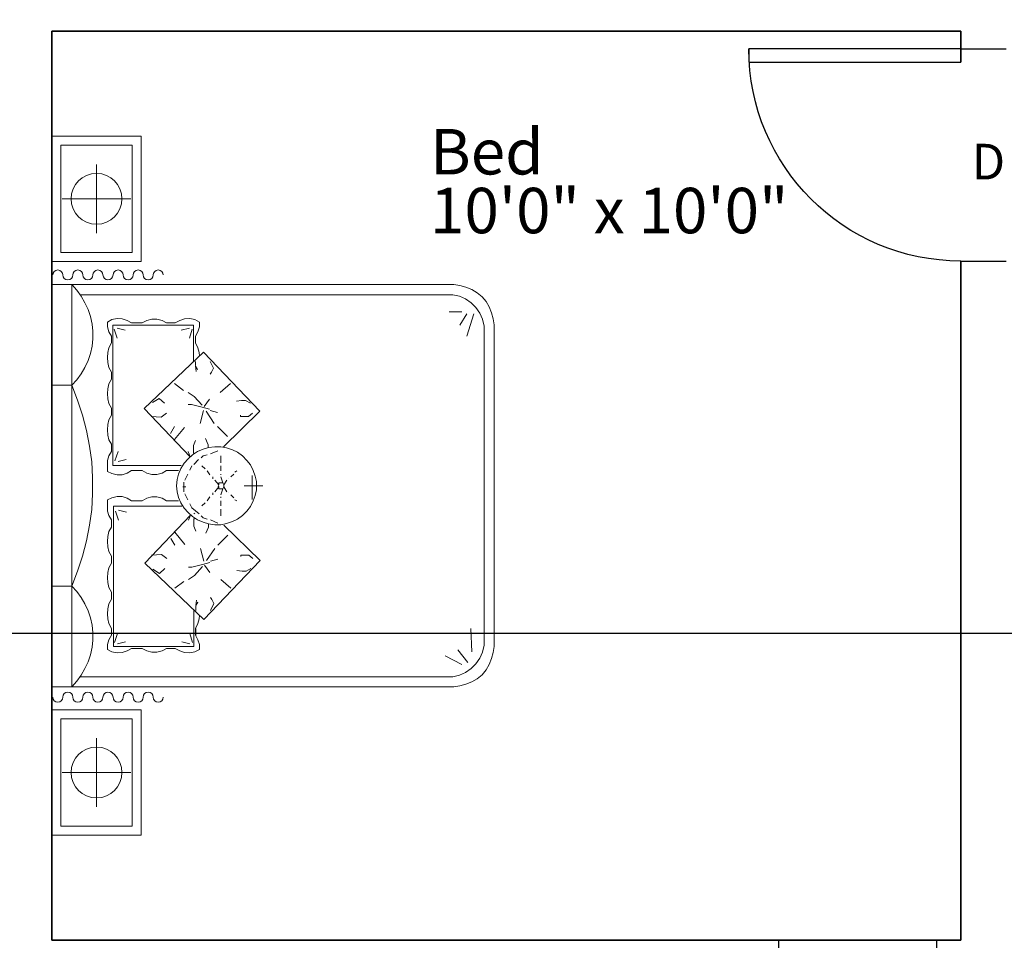
# Model space of a CAD drawing. Units: inches. Extents: x -1198 to -69, y -512 to 437.
# Tile 27 of 50: x -696 to -566, y -85 to 37. Entities that reach past the tile are written whole.
import ezdxf

# ---------------------------------------------------------------- set-up
doc = ezdxf.new("R2010")
doc.units = ezdxf.units.IN
doc.header["$MEASUREMENT"] = 0
for name, color, linetype, lineweight in [('A-ANNO-DIMS', 2, 'Continuous', 18), ('A-ANNO-SYMB', 7, 'Continuous', 18), ('A-AREA-IDEN', 7, 'Continuous', 18), ('A-FURN', 60, 'Continuous', 18), ('A-WALL', 7, 'Continuous', 35), ('Doors', 140, 'Continuous', 25), ('ds_furniture_Pen_No__7', 7, 'Continuous', 18)]:
    doc.layers.add(name, color=color, linetype=linetype, lineweight=lineweight)
doc.styles.get("Standard").update_dxf_attribs({"font": 'arial.ttf'})
doc.dimstyles.get("Standard").update_dxf_attribs({"dimtxt": 6, "dimasz": 6, "dimexe": 0.18, "dimexo": 0.0625, "dimgap": 0.09, "dimtad": 0, "dimtih": 1, "dimtoh": 1, "dimdec": 0, "dimzin": 0, "dimdsep": 46, "dimlunit": 4, "dimtxsty": 'Standard', "dimblk": 'OBLIQUE', "dimcen": 0.09, "dimadec": 0, "dimazin": 0, "dimtfac": 1, "dimtdec": 0, "dimtofl": 0, "dimtmove": 0, "dimatfit": 3, "dimfxl": 1, "dimtolj": 1, "dimtzin": 0, "dimarcsym": 0})

# ---------------------------------------------------------------- blocks, each defined once
blk = doc.blocks.new('*U4')
for p, q in [((0, 0), (0, -6)), ((28, 0), (28, -6))]:
    blk.add_line(p, q)
blk.add_lwpolyline([(0, 0), (0, 28), (1.75, 28), (1.75, 0)], close=True)
blk.add_arc((0, 0), 28, 0, 90)
blk = doc.blocks.new('new')
at = {"layer": 'ds_furniture_Pen_No__7'}
for p, q in [((-1180, 2274.4), (-1838.2, 2274.4)), ((-1838.2, 2274.4), (-1838.2, 1804.2)), ((-1180, 1804.2), (-1180, 2274.4)), ((-1057.8, 158.7), (-1057.8, 2274.4)), ((-1057.8, 2274.4), (1057.8, 2274.4)), ((-1057.8, 2274.4), (1057.8, 2274.4)), ((-1057.8, 158.7), (-1057.8, 2274.4)), ((-528.9, 2274.4), (-528.9, 2168.6)), ((528.9, 2274.4), (528.9, 2168.6)), ((1057.8, 2274.4), (1057.8, 158.7)), ((1057.8, 2274.4), (1057.8, 158.7)), ((1180, 1804.2), (1180, 2274.4)), ((1180, 2274.4), (1838.2, 2274.4)), ((1838.2, 2274.4), (1838.2, 1804.2)), ((-1227, 2227.4), (-1791.2, 2227.4)), ((-1791.2, 2227.4), (-1791.2, 1851.2)), ((-1509.1, 2220.2), (-1509.1, 1858.4)), ((-1227, 1851.2), (-1227, 2227.4)), ((1227, 1851.2), (1227, 2227.4)), ((1227, 2227.4), (1791.2, 2227.4)), ((1509.1, 2220.2), (1509.1, 1858.4)), ((1791.2, 2227.4), (1791.2, 1851.2)), ((1057.8, 2168.6), (-1057.8, 2168.6)), ((-1057.8, 2168.6), (-1028.2, 2143.2)), ((-1028.2, 2143.2), (-996.5, 2119.9)), ((-588.2, 2119.9), (-556.4, 2143.2)), ((-556.4, 2143.2), (-528.9, 2168.6)), ((-528.9, 2168.6), (-450.6, 2139)), ((-450.6, 2139), (-370.2, 2113.6)), ((370.2, 2113.6), (450.6, 2139)), ((450.6, 2139), (528.9, 2168.6)), ((528.9, 2168.6), (556.4, 2143.2)), ((556.4, 2143.2), (588.2, 2119.9)), ((996.5, 2119.9), (1028.2, 2143.2)), ((1028.2, 2143.2), (1057.8, 2168.6)), ((-1005, 165), (-1005, 2124.2)), ((-996.5, 2119.9), (-962.6, 2100.9)), ((-962.6, 2100.9), (-926.7, 2084)), ((-926.7, 2084), (-890.7, 2071.3)), ((-696.1, 2071.3), (-658, 2084)), ((-658, 2084), (-622, 2100.9)), ((-622, 2100.9), (-588.2, 2119.9)), ((-370.2, 2113.6), (-289.9, 2092.4)), ((-289.9, 2092.4), (-207.3, 2075.5)), ((-207.3, 2075.5), (-124.8, 2064.9)), ((124.8, 2064.9), (207.3, 2075.5)), ((207.3, 2075.5), (289.9, 2092.4)), ((289.9, 2092.4), (370.2, 2113.6)), ((588.2, 2119.9), (622, 2100.9)), ((622, 2100.9), (658, 2084)), ((658, 2084), (696.1, 2071.3)), ((890.7, 2071.3), (926.7, 2084)), ((926.7, 2084), (962.6, 2100.9)), ((962.6, 2100.9), (996.5, 2119.9)), ((1005, 2124.2), (1005, 165)), ((-1690.1, 2039.3), (-1328.2, 2039.3)), ((-890.7, 2071.3), (-850.5, 2062.8)), ((-850.5, 2062.8), (-812.4, 2058.6)), ((-812.4, 2058.6), (-772.2, 2058.6)), ((-772.2, 2058.6), (-734.1, 2062.8)), ((-734.1, 2062.8), (-696.1, 2071.3)), ((-124.8, 2064.9), (-42.3, 2060.7)), ((-42.3, 2060.7), (42.3, 2060.7)), ((42.3, 2060.7), (124.8, 2064.9)), ((696.1, 2071.3), (734.1, 2062.8)), ((734.1, 2062.8), (772.2, 2058.6)), ((772.2, 2058.6), (812.4, 2058.6)), ((812.4, 2058.6), (850.5, 2062.8)), ((850.5, 2062.8), (890.7, 2071.3)), ((1690.1, 2039.3), (1328.2, 2039.3)), ((-873.8, 1959.1), (-861.1, 1982.4)), ((-861.1, 1982.4), (-835.7, 1982.4)), ((-835.7, 1982.4), (-810.3, 1973.9)), ((-810.3, 1973.9), (-787, 1961.2)), ((-751.1, 1961.2), (-725.7, 1973.9)), ((-725.7, 1973.9), (-700.3, 1980.3)), ((-700.3, 1980.3), (-674.9, 1982.4)), ((-674.9, 1982.4), (-647.4, 1980.3)), ((-647.4, 1980.3), (-622, 1973.9)), ((-622, 1973.9), (-596.6, 1961.2)), ((-560.7, 1961.2), (-535.3, 1973.9)), ((-535.3, 1973.9), (-509.9, 1980.3)), ((-509.9, 1980.3), (-484.5, 1982.4)), ((-484.5, 1982.4), (-457, 1980.3)), ((-457, 1980.3), (-431.6, 1973.9)), ((-431.6, 1973.9), (-408.3, 1961.2)), ((-370.2, 1961.2), (-347, 1973.9)), ((-347, 1973.9), (-321.6, 1980.3)), ((-321.6, 1980.3), (-294.1, 1982.4)), ((-294.1, 1982.4), (-266.6, 1980.3)), ((-266.6, 1980.3), (-241.2, 1973.9)), ((-241.2, 1973.9), (-217.9, 1961.2)), ((-179.8, 1961.2), (-156.6, 1973.9)), ((-156.6, 1973.9), (-133.3, 1982.4)), ((-133.3, 1982.4), (-105.8, 1982.4)), ((-105.8, 1982.4), (-74, 1982.4)), ((-74, 1982.4), (-63.5, 1959.1)), ((74, 1982.4), (63.5, 1959.1)), ((105.8, 1982.4), (74, 1982.4)), ((133.3, 1982.4), (105.8, 1982.4)), ((156.6, 1973.9), (133.3, 1982.4)), ((179.8, 1961.2), (156.6, 1973.9)), ((241.2, 1973.9), (217.9, 1961.2)), ((266.6, 1980.3), (241.2, 1973.9)), ((294.1, 1982.4), (266.6, 1980.3)), ((321.6, 1980.3), (294.1, 1982.4)), ((347, 1973.9), (321.6, 1980.3)), ((370.2, 1961.2), (347, 1973.9)), ((431.6, 1973.9), (408.3, 1961.2)), ((457, 1980.3), (431.6, 1973.9)), ((484.5, 1982.4), (457, 1980.3)), ((509.9, 1980.3), (484.5, 1982.4)), ((535.3, 1973.9), (509.9, 1980.3)), ((560.7, 1961.2), (535.3, 1973.9)), ((622, 1973.9), (596.6, 1961.2)), ((647.4, 1980.3), (622, 1973.9)), ((674.9, 1982.4), (647.4, 1980.3)), ((700.3, 1980.3), (674.9, 1982.4)), ((725.7, 1973.9), (700.3, 1980.3)), ((751.1, 1961.2), (725.7, 1973.9)), ((810.3, 1973.9), (787, 1961.2)), ((835.7, 1982.4), (810.3, 1973.9)), ((861.1, 1982.4), (835.7, 1982.4)), ((873.8, 1959.1), (861.1, 1982.4)), ((-880.1, 1931.6), (-873.8, 1959.1)), ((-878, 1904.1), (-880.1, 1931.6)), ((-846.3, 1527.5), (-846.3, 1950.7)), ((-846.3, 1950.7), (-107.9, 1950.7)), ((-831.5, 1929.5), (-820.9, 1887.2)), ((-825.1, 1944.3), (-778.6, 1929.5)), ((-787, 1961.2), (-751.1, 1961.2)), ((-596.6, 1961.2), (-560.7, 1961.2)), ((-408.3, 1961.2), (-370.2, 1961.2)), ((-217.9, 1961.2), (-179.8, 1961.2)), ((-133.3, 1940.1), (-181.9, 1923.2)), ((-129.1, 1923.2), (-139.6, 1880.9)), ((-107.9, 1950.7), (-107.9, 1591)), ((-63.5, 1959.1), (-57.1, 1931.6)), ((-57.1, 1931.6), (-57.1, 1904.1)), ((63.5, 1959.1), (57.1, 1931.6)), ((57.1, 1931.6), (57.1, 1904.1)), ((844.2, 1952.8), (105.8, 1952.8)), ((105.8, 1952.8), (105.8, 1593.1)), ((126.9, 1925.3), (137.5, 1883)), ((131.2, 1942.2), (179.8, 1925.3)), ((217.9, 1961.2), (179.8, 1961.2)), ((408.3, 1961.2), (370.2, 1961.2)), ((596.6, 1961.2), (560.7, 1961.2)), ((787, 1961.2), (751.1, 1961.2)), ((823, 1946.4), (776.5, 1931.6)), ((829.4, 1931.6), (818.8, 1889.3)), ((844.2, 1529.6), (844.2, 1952.8)), ((880.1, 1931.6), (873.8, 1959.1)), ((878, 1904.1), (880.1, 1931.6)), ((-869.6, 1878.7), (-878, 1904.1)), ((-856.9, 1855.5), (-869.6, 1878.7)), ((-65.6, 1878.7), (-80.4, 1855.5)), ((-57.1, 1904.1), (-65.6, 1878.7)), ((57.1, 1904.1), (65.6, 1878.7)), ((65.6, 1878.7), (80.4, 1855.5)), ((856.9, 1855.5), (869.6, 1878.7)), ((869.6, 1878.7), (878, 1904.1)), ((-1791.2, 1851.2), (-1227, 1851.2)), ((-856.9, 1798.3), (-856.9, 1855.5)), ((-80.4, 1855.5), (-80.4, 1798.3)), ((80.4, 1855.5), (80.4, 1798.3)), ((856.9, 1798.3), (856.9, 1855.5)), ((1791.2, 1851.2), (1227, 1851.2)), ((-1838.2, 1804.2), (-1180, 1804.2)), ((-875.9, 1747.6), (-869.6, 1775.1)), ((-869.6, 1775.1), (-856.9, 1798.3)), ((-704.5, 1474.6), (-408.3, 1785.6)), ((-408.3, 1785.6), (-154.4, 1544.5)), ((-80.4, 1798.3), (-65.6, 1775.1)), ((-65.6, 1775.1), (-59.2, 1747.6)), ((65.6, 1775.1), (59.2, 1747.6)), ((80.4, 1798.3), (65.6, 1775.1)), ((406.2, 1787.8), (152.3, 1546.6)), ((702.4, 1476.8), (406.2, 1787.8)), ((869.6, 1775.1), (856.9, 1798.3)), ((875.9, 1747.6), (869.6, 1775.1)), ((1838.2, 1804.2), (1180, 1804.2)), ((-875.9, 1722.2), (-875.9, 1747.6)), ((-869.6, 1694.7), (-875.9, 1722.2)), ((-440.1, 1743.3), (-461.2, 1707.4)), ((-366, 1749.7), (-361.8, 1696.8)), ((-59.2, 1722.2), (-65.6, 1694.7)), ((-59.2, 1747.6), (-59.2, 1722.2)), ((59.2, 1747.6), (59.2, 1722.2)), ((59.2, 1722.2), (65.6, 1694.7)), ((363.9, 1751.8), (359.7, 1698.9)), ((437.9, 1745.4), (459.1, 1709.5)), ((869.6, 1694.7), (875.9, 1722.2)), ((875.9, 1722.2), (875.9, 1747.6)), ((-856.9, 1671.4), (-869.6, 1694.7)), ((-856.9, 1624.9), (-856.9, 1671.4)), ((-461.2, 1707.4), (-435.8, 1679.9)), ((-361.8, 1696.8), (-382.9, 1669.3)), ((-65.6, 1694.7), (-80.4, 1671.4)), ((-80.4, 1671.4), (-80.4, 1607.9)), ((65.6, 1694.7), (80.4, 1671.4)), ((80.4, 1671.4), (80.4, 1607.9)), ((359.7, 1698.9), (380.8, 1671.4)), ((459.1, 1709.5), (433.7, 1682)), ((856.9, 1671.4), (869.6, 1694.7)), ((856.9, 1624.9), (856.9, 1671.4)), ((-869.6, 1601.6), (-856.9, 1624.9)), ((-539.5, 1627), (-503.5, 1580.4)), ((-277.2, 1648.1), (-313.1, 1627)), ((-245.4, 1627), (-308.9, 1574.1)), ((-91, 1595.2), (-61.4, 1607.9)), ((-61.4, 1607.9), (-31.7, 1614.3)), ((-31.7, 1614.3), (0, 1618.5)), ((0, 1618.5), (31.7, 1614.3)), ((31.7, 1614.3), (61.4, 1607.9)), ((61.4, 1607.9), (91, 1595.2)), ((243.3, 1629.1), (306.8, 1576.2)), ((275, 1650.2), (311, 1629.1)), ((537.4, 1629.1), (501.4, 1582.5)), ((869.6, 1601.6), (856.9, 1624.9)), ((-880.1, 1548.7), (-878, 1576.2)), ((-878, 1576.2), (-869.6, 1601.6)), ((-831.5, 1548.7), (-820.9, 1591)), ((-471.8, 1523.3), (-493, 1555)), ((-429.5, 1538.1), (-429.5, 1555)), ((-181.9, 1555), (-154.4, 1544.5)), ((-162.9, 1533.9), (-141.8, 1557.2)), ((-141.8, 1557.2), (-118.5, 1578.3)), ((-118.5, 1578.3), (-91, 1595.2)), ((-42.3, 1574.1), (-74, 1559.3)), ((-31.7, 1580.4), (-2.1, 1580.4)), ((19, 1580.4), (-10.6, 1580.4)), ((-6.3, 1584.7), (-6.3, 1569.8)), ((-6.3, 1584.7), (-6.3, 1569.8)), ((29.6, 1574.1), (61.4, 1559.3)), ((91, 1595.2), (118.5, 1578.3)), ((118.5, 1578.3), (141.8, 1557.2)), ((141.8, 1557.2), (162.9, 1533.9)), ((179.8, 1557.2), (152.3, 1546.6)), ((427.4, 1540.2), (427.4, 1557.2)), ((469.7, 1525.4), (490.8, 1557.2)), ((829.4, 1550.8), (818.8, 1593.1)), ((878, 1576.2), (869.6, 1601.6)), ((880.1, 1548.7), (878, 1576.2)), ((-873.8, 1521.2), (-880.1, 1548.7)), ((-861.1, 1497.9), (-873.8, 1521.2)), ((-651.6, 1527.5), (-846.3, 1527.5)), ((-810.3, 1506.4), (-835.7, 1497.9)), ((-825.1, 1533.9), (-778.6, 1548.7)), ((-787, 1519.1), (-810.3, 1506.4)), ((-772.2, 1517), (-789.2, 1517)), ((-751.1, 1519.1), (-787, 1519.1)), ((-761.7, 1517), (-772.2, 1517)), ((-751.1, 1517), (-761.7, 1517)), ((-725.7, 1506.4), (-751.1, 1519.1)), ((-700.3, 1500), (-725.7, 1506.4)), ((-655.9, 1517), (-634.7, 1517)), ((-634.7, 1517), (-613.6, 1506.4)), ((-613.6, 1506.4), (-630.5, 1517)), ((-630.5, 1517), (-603, 1512.7)), ((-425.3, 1481), (-471.8, 1523.3)), ((-414.7, 1481), (-429.5, 1538.1)), ((-213.7, 1527.5), (-239.1, 1517)), ((-175.6, 1527.5), (-213.7, 1527.5)), ((-192.5, 1478.9), (-179.8, 1508.5)), ((-179.8, 1508.5), (-162.9, 1533.9)), ((-175.6, 1527.5), (-171.4, 1523.3)), ((-116.4, 1538.1), (-148.1, 1500)), ((-148.1, 1527.5), (-143.9, 1521.2)), ((-116.4, 1538.1), (-95.2, 1548.7)), ((103.7, 1538.1), (82.5, 1548.7)), ((112.1, 1527.5), (137.5, 1502.1)), ((162.9, 1533.9), (179.8, 1508.5)), ((173.5, 1529.6), (169.3, 1525.4)), ((173.5, 1529.6), (211.6, 1529.6)), ((179.8, 1508.5), (192.5, 1478.9)), ((211.6, 1529.6), (237, 1519.1)), ((412.6, 1483.1), (427.4, 1540.2)), ((423.1, 1483.1), (469.7, 1525.4)), ((628.4, 1519.1), (600.9, 1514.8)), ((632.6, 1519.1), (611.4, 1508.5)), ((611.4, 1508.5), (628.4, 1519.1)), ((653.7, 1519.1), (632.6, 1519.1)), ((649.5, 1529.6), (844.2, 1529.6)), ((700.3, 1500), (725.7, 1506.4)), ((725.7, 1506.4), (751.1, 1519.1)), ((749, 1519.1), (759.5, 1519.1)), ((751.1, 1519.1), (787, 1519.1)), ((759.5, 1519.1), (770.1, 1519.1)), ((770.1, 1519.1), (787, 1519.1)), ((823, 1536), (776.5, 1550.8)), ((787, 1519.1), (810.3, 1506.4)), ((810.3, 1506.4), (835.7, 1497.9)), ((861.1, 1497.9), (873.8, 1521.2)), ((873.8, 1521.2), (880.1, 1548.7)), ((-835.7, 1497.9), (-861.1, 1497.9)), ((-393.5, 1178.4), (-704.5, 1474.6)), ((-683.4, 1497.9), (-700.3, 1500)), ((-457, 1442.9), (-418.9, 1470.4)), ((-404.1, 1442.9), (-414.7, 1481)), ((-397.8, 1474.6), (-330, 1491.6)), ((-393.5, 1459.8), (-330, 1417.5)), ((-217.9, 1449.3), (-249.7, 1464.1)), ((-201, 1449.3), (-192.5, 1478.9)), ((-169.3, 1478.9), (-175.6, 1457.7)), ((-169.3, 1478.9), (-158.7, 1489.4)), ((-91, 1468.3), (-105.8, 1485.2)), ((-59.2, 1442.9), (-80.4, 1457.7)), ((57.1, 1442.9), (78.3, 1457.7)), ((88.9, 1468.3), (103.7, 1485.2)), ((156.6, 1478.9), (146, 1489.4)), ((156.6, 1478.9), (162.9, 1457.7)), ((192.5, 1478.9), (201, 1449.3)), ((215.8, 1451.4), (201, 1451.4)), ((215.8, 1451.4), (247.5, 1466.2)), ((395.6, 1476.8), (327.9, 1493.7)), ((391.4, 1461.9), (327.9, 1419.6)), ((391.4, 1180.6), (702.4, 1476.8)), ((402, 1445), (412.6, 1483.1)), ((454.9, 1445), (416.8, 1472.5)), ((683.4, 1497.9), (700.3, 1500)), ((835.7, 1497.9), (861.1, 1497.9)), ((-655.9, 1438.7), (-619.9, 1421.7)), ((-619.9, 1421.7), (-598.7, 1432.3)), ((-598.7, 1432.3), (-588.2, 1438.7)), ((-397.8, 1438.7), (-387.2, 1400.6)), ((-260.2, 1347.7), (-313.1, 1400.6)), ((-217.9, 1449.3), (-203.1, 1449.3)), ((-205.2, 1417.5), (-201, 1449.3)), ((-205.2, 1385.8), (-205.2, 1417.5)), ((-196.8, 1400.6), (-179.8, 1438.7)), ((-38.1, 1428.1), (-48.7, 1428.1)), ((-6.3, 1396.4), (-31.7, 1417.5)), ((4.2, 1396.4), (29.6, 1417.5)), ((36, 1428.1), (46.5, 1428.1)), ((184.1, 1400.6), (167.1, 1438.7)), ((201, 1449.3), (205.2, 1417.5)), ((205.2, 1417.5), (205.2, 1385.8)), ((258.1, 1349.8), (311, 1402.7)), ((395.6, 1440.8), (385.1, 1402.7)), ((596.6, 1434.4), (586, 1440.8)), ((617.8, 1423.9), (596.6, 1434.4)), ((653.7, 1440.8), (617.8, 1423.9)), ((-539.5, 1332.9), (-493, 1385.8)), ((-393.5, 1178.4), (-207.3, 1368.9)), ((-198.9, 1356.2), (-205.2, 1385.8)), ((-188.3, 1324.4), (-198.9, 1356.2)), ((-122.7, 1385.8), (-158.7, 1385.8)), ((-80.4, 1385.8), (-105.8, 1385.8)), ((-59.2, 1385.8), (-63.5, 1385.8)), ((-16.9, 1375.2), (-48.7, 1385.8)), ((-6.3, 1368.9), (-31.7, 1354)), ((-16.9, 1385.8), (-16.9, 1396.4)), ((-16.9, 1396.4), (-6.3, 1396.4)), ((-16.9, 1375.2), (-16.9, 1385.8)), ((-6.3, 1368.9), (-16.9, 1375.2)), ((-6.3, 1396.4), (-2.1, 1398.5)), ((-6.3, 1368.9), (-2.1, 1368.9)), ((4.2, 1396.4), (-2.1, 1398.5)), ((4.2, 1368.9), (-2.1, 1368.9)), ((14.8, 1396.4), (4.2, 1396.4)), ((4.2, 1368.9), (14.8, 1375.2)), ((4.2, 1368.9), (29.6, 1354)), ((14.8, 1385.8), (14.8, 1396.4)), ((14.8, 1375.2), (14.8, 1385.8)), ((14.8, 1375.2), (46.5, 1385.8)), ((57.1, 1385.8), (61.4, 1385.8)), ((78.3, 1385.8), (103.7, 1385.8)), ((120.6, 1385.8), (156.6, 1385.8)), ((198.9, 1356.2), (188.3, 1324.4)), ((205.2, 1385.8), (198.9, 1356.2)), ((391.4, 1180.6), (205.2, 1371)), ((537.4, 1335), (490.8, 1387.9)), ((-450.6, 1273.6), (-446.4, 1301.2)), ((-175.6, 1296.9), (-188.3, 1324.4)), ((-156.6, 1271.5), (-175.6, 1296.9)), ((-74, 1311.7), (-80.4, 1301.2)), ((-48.7, 1332.9), (-63.5, 1316)), ((-38.1, 1343.5), (-38, 1343.5)), ((36, 1343.5), (36, 1343.5)), ((46.5, 1332.9), (61.4, 1316)), ((71.9, 1311.7), (78.3, 1301.2)), ((175.6, 1296.9), (156.6, 1271.5)), ((188.3, 1324.4), (175.6, 1296.9)), ((448.5, 1275.8), (444.3, 1303.3)), ((-450.6, 1252.5), (-450.6, 1273.6)), ((-435.8, 1227.1), (-450.6, 1252.5)), ((-366, 1280), (-372.4, 1280)), ((-366, 1237.7), (-366, 1280)), ((-133.3, 1248.3), (-156.6, 1271.5)), ((-110, 1229.2), (-133.3, 1248.3)), ((0, 1163.6), (0, 1263.1)), ((133.3, 1248.3), (110, 1229.2)), ((156.6, 1271.5), (133.3, 1248.3)), ((363.9, 1239.8), (363.9, 1282.1)), ((363.9, 1282.1), (370.2, 1282.1)), ((433.7, 1229.2), (448.5, 1254.6)), ((448.5, 1254.6), (448.5, 1275.8)), ((-382.9, 1216.5), (-366, 1237.7)), ((-80.4, 1214.4), (-110, 1229.2)), ((-50.8, 1203.8), (-80.4, 1214.4)), ((52.9, 1220.8), (-71.9, 1220.8)), ((-21.2, 1197.5), (-50.8, 1203.8)), ((0, 1197.5), (-21.2, 1197.5)), ((21.2, 1197.5), (0, 1197.5)), ((50.8, 1203.8), (21.2, 1197.5)), ((80.4, 1214.4), (50.8, 1203.8)), ((110, 1229.2), (80.4, 1214.4)), ((380.8, 1218.6), (363.9, 1239.8)), ((-1053.6, 126.9), (-1057.8, 158.7)), ((-1053.6, 126.9), (-1057.8, 158.7)), ((-996.5, 129.1), (-1005, 165)), ((-941.5, 116.4), (-894.9, 205.2)), ((914, 116.4), (914, 184.1)), ((1005, 165), (996.5, 129.1)), ((1057.8, 158.7), (1053.6, 126.9)), ((1057.8, 158.7), (1053.6, 126.9)), ((-1045.2, 95.2), (-1053.6, 126.9)), ((-1045.2, 95.2), (-1053.6, 126.9)), ((-983.8, 97.3), (-996.5, 129.1)), ((-930.9, 84.6), (-863.2, 137.5)), ((903.4, 91), (844.2, 126.9)), ((996.5, 129.1), (983.8, 97.3)), ((1053.6, 126.9), (1045.2, 95.2)), ((1053.6, 126.9), (1045.2, 95.2)), ((-1032.5, 63.5), (-1045.2, 95.2)), ((-1032.5, 63.5), (-1045.2, 95.2)), ((-1015.5, 36), (-1032.5, 63.5)), ((-1015.5, 36), (-1032.5, 63.5)), ((-962.6, 67.7), (-983.8, 97.3)), ((-937.3, 42.3), (-962.6, 67.7)), ((-873.8, 63.5), (-751.1, 69.8)), ((903.4, 52.9), (787, 91)), ((962.6, 67.7), (937.3, 42.3)), ((983.8, 97.3), (962.6, 67.7)), ((1032.5, 63.5), (1015.5, 36)), ((1032.5, 63.5), (1015.5, 36)), ((1045.2, 95.2), (1032.5, 63.5)), ((1045.2, 95.2), (1032.5, 63.5)), ((-994.4, 10.6), (-1015.5, 36)), ((-994.4, 10.6), (-1015.5, 36)), ((-969, -10.6), (-994.4, 10.6)), ((-969, -10.6), (-994.4, 10.6)), ((-907.6, 21.2), (-937.3, 42.3)), ((-875.9, 8.5), (-907.6, 21.2)), ((-839.9, 0), (-875.9, 8.5)), ((839.9, 0), (-839.9, 0)), ((875.9, 8.5), (839.9, 0)), ((907.6, 21.2), (875.9, 8.5)), ((937.3, 42.3), (907.6, 21.2)), ((994.4, 10.6), (969, -10.6)), ((994.4, 10.6), (969, -10.6)), ((1015.5, 36), (994.4, 10.6)), ((1015.5, 36), (994.4, 10.6)), ((-941.5, -27.5), (-969, -10.6)), ((-941.5, -27.5), (-969, -10.6)), ((-909.7, -40.2), (-941.5, -27.5)), ((-909.7, -40.2), (-941.5, -27.5)), ((-878, -48.7), (-909.7, -40.2)), ((-878, -48.7), (-909.7, -40.2)), ((-846.3, -52.9), (-878, -48.7)), ((-846.3, -52.9), (-878, -48.7)), ((878, -48.7), (846.3, -52.9)), ((878, -48.7), (846.3, -52.9)), ((909.7, -40.2), (878, -48.7)), ((909.7, -40.2), (878, -48.7)), ((941.5, -27.5), (909.7, -40.2)), ((941.5, -27.5), (909.7, -40.2)), ((969, -10.6), (941.5, -27.5)), ((969, -10.6), (941.5, -27.5)), ((846.3, -52.9), (-846.3, -52.9)), ((846.3, -52.9), (-846.3, -52.9))]:
    blk.add_line(p, q, dxfattribs=at)
for centre in [(-1509.1, 2039.3), (1509.1, 2039.3)]:
    blk.add_circle(centre, 133.9, dxfattribs=at)
for centre, start, end in [((-1112.8, 2243.5), 90, 270), ((1108.7, 2243.5), 270, 90), ((-1112.8, 2190.6), 270, 90), ((1108.7, 2190.6), 90, 270), ((-1112.8, 2137.7), 90, 270), ((1108.7, 2137.7), 270, 90), ((-1112.8, 2084.8), 270, 90), ((-1112.8, 2084.8), 270, 90), ((1108.7, 2084.8), 90, 270), ((1108.7, 2084.8), 90, 270), ((-1112.8, 2031.9), 90, 270), ((1108.7, 2031.9), 270, 90), ((-1112.8, 1979), 270, 90), ((1108.7, 1979), 90, 270), ((-1112.8, 1926.1), 90, 270), ((1108.7, 1926.1), 270, 90), ((-1112.8, 1873.2), 270, 90), ((1108.7, 1873.2), 90, 270), ((-1112.8, 1820.3), 90, 270), ((1108.7, 1820.3), 270, 90), ((-1112.8, 1767.4), 270, 90), ((1108.7, 1767.4), 90, 270), ((-1112.8, 1714.6), 90, 270), ((1108.7, 1714.6), 270, 90)]:
    blk.add_arc(centre, 26.4, start, end, dxfattribs=at)
blk = doc.blocks.new('DOOR-D1-JAMB3')
for p, q in [((0, 0), (0, -3)), ((20.87, 0), (20.87, -3))]:
    blk.add_line(p, q)
blk.add_lwpolyline([(0, 0), (0, 20.87), (1.3, 20.87), (1.3, 0)], close=True)
blk.add_arc((0, 0), 20.87, 0, 90)
blk = doc.blocks.new('_Oblique')
at = {"color": 0, "linetype": 'ByBlock', "lineweight": -2}
blk.add_line((-0.5, -0.5), (0.5, 0.5), dxfattribs=at)
blk = doc.blocks.new('*D75')
at = {"layer": 'A-ANNO-DIMS', "color": 0, "lineweight": -2, "ltscale": 10, "transparency": 16777216}
for p, q in [((-376.81, -44.27), (-1188.2, -44.27)), ((-1188.02, -44.27), (-1188.02, -133.37)), ((-1188.02, -228.77), (-1188.02, -139.68)), ((-370.81, -228.77), (-1188.2, -228.77))]:
    blk.add_line(p, q, dxfattribs=at)
at = {"layer": 'DEFPOINTS', "color": 0, "ltscale": 10, "transparency": 16777216}
for p in [(-1188.02, -44.27), (-376.75, -44.27), (-370.75, -228.77)]:
    blk.add_point(p, dxfattribs=at)
at = {"layer": 'A-ANNO-DIMS', "color": 0, "lineweight": -2, "ltscale": 10, "transparency": 16777216, "xscale": 6, "yscale": 6, "zscale": 6}
for p, rotation in [((-1188.02, -44.27), 90), ((-1188.02, -228.77), 270)]:
    blk.add_blockref('_Oblique', p, dxfattribs=dict(at, rotation=rotation))
at = {"layer": 'A-ANNO-DIMS', "color": 0, "ltscale": 10, "transparency": 16777216, "insert": (-1188.02, -136.52), "char_height": 6, "attachment_point": 5}
blk.add_mtext('\\A1;184.5', dxfattribs=at)
blk = doc.blocks.new('*D76')
at = {"layer": 'A-ANNO-DIMS', "color": 0, "lineweight": -2, "ltscale": 10, "transparency": 16777216}
for p, q in [((-711.13, -38.21), (-711.13, 433.18)), ((-711.13, 433), (-697.75, 433)), ((-697.75, -38.21), (-697.75, 433.18)), ((-697.75, 433), (-691.75, 433))]:
    blk.add_line(p, q, dxfattribs=at)
at = {"layer": 'DEFPOINTS', "color": 0, "ltscale": 10, "transparency": 16777216}
for p in [(-697.75, 433), (-711.13, -38.27), (-697.75, -38.27)]:
    blk.add_point(p, dxfattribs=at)
at = {"layer": 'A-ANNO-DIMS', "color": 0, "lineweight": -2, "ltscale": 10, "transparency": 16777216, "xscale": 6, "yscale": 6, "zscale": 6, "rotation": 180}
blk.add_blockref('_Oblique', (-711.13, 433), dxfattribs=at)
at = {"layer": 'A-ANNO-DIMS', "color": 0, "lineweight": -2, "ltscale": 10, "transparency": 16777216, "xscale": 6, "yscale": 6, "zscale": 6}
blk.add_blockref('_Oblique', (-697.75, 433), dxfattribs=at)
at = {"layer": 'A-ANNO-DIMS', "color": 0, "ltscale": 10, "transparency": 16777216, "insert": (-681.81, 433), "char_height": 6, "attachment_point": 5}
blk.add_mtext('\\A1;13.38', dxfattribs=at)

msp = doc.modelspace()

# ---------------------------------------------------------------- linework, layer by layer
at = {"layer": 'A-WALL', "ltscale": 10}
for p, q in [((-571.7509, 35.2277), (-691.7509, 35.2277)), ((-691.7509, 35.2277), (-691.7509, -84.7723)), ((-691.7509, 35.2277), (-691.7509, -84.7723)), ((-571.7509, 35.2277), (-571.7509, 31.124)), ((-571.7509, 4.874), (-571.7509, -84.7723)), ((-571.7509, -84.7723), (-691.7509, -84.7723))]:
    msp.add_line(p, q, dxfattribs=at)

# ---------------------------------------------------------------- block references
at = {"layer": 'A-FURN', "xscale": 0.0250833463801972, "yscale": 0.0250833463801972, "zscale": 0.0250833463801972, "rotation": 90}
msp.add_blockref('new', (-634.702, -24.7723), dxfattribs=at)
at = {"layer": 'Doors', "xscale": -1, "rotation": 90}
msp.add_blockref('*U4', (-571.7509, 32.874), dxfattribs=at)
at = {"layer": 'Doors', "rotation": 180}
msp.add_blockref('DOOR-D1-JAMB3', (-574.9123, -87.7723), dxfattribs=at)

# ---------------------------------------------------------------- texts
at = {"layer": 'A-ANNO-SYMB', "ltscale": 10}
msp.add_text('D', height=4.6996, dxfattribs=at).set_placement((-570.3184, 15.6475))
at = {"layer": 'A-AREA-IDEN', "ltscale": 10, "char_height": 6, "attachment_point": 1}
for s, insert in [('Bed', (-641.8292, 22.3036)), ('10\'0" x 10\'0"', (-641.8292, 14.5396))]:
    msp.add_mtext_dynamic_manual_height_columns(s, width=57.976527, gutter_width=30, heights=[0], dxfattribs=dict(at, insert=insert))

# ---------------------------------------------------------------- dimensions: what is measured, and where the dimension line sits
at = {"layer": 'A-ANNO-DIMS', "ltscale": 10}
dim = msp.add_linear_dim(base=(-697.7509, 433.0036), p1=(-711.1319, -38.2723), p2=(-697.7509, -38.2723), dimstyle='Standard', override={"dimdec": 2, "dimlfac": 1, "dimrnd": 0, "dimzin": 0, "dimdsep": 46, "dimlunit": 2}, dxfattribs=at)
dim.commit()
dim.dimension.update_dxf_attribs({"geometry": '*D76', "text_midpoint": (-681.8137, 433.0036)})
dim = msp.add_linear_dim(base=(-1188.0248, -44.2723), p1=(-370.7509, -228.7723), p2=(-376.7509, -44.2723), angle=90, dimstyle='Standard', override={"dimdec": 1, "dimlfac": 1, "dimrnd": 0, "dimzin": 0, "dimdsep": 46, "dimlunit": 2}, dxfattribs=at)
dim.commit()
dim.dimension.update_dxf_attribs({"geometry": '*D75', "text_midpoint": (-1188.0248, -136.5223)})

doc.saveas('drawing.dxf')
